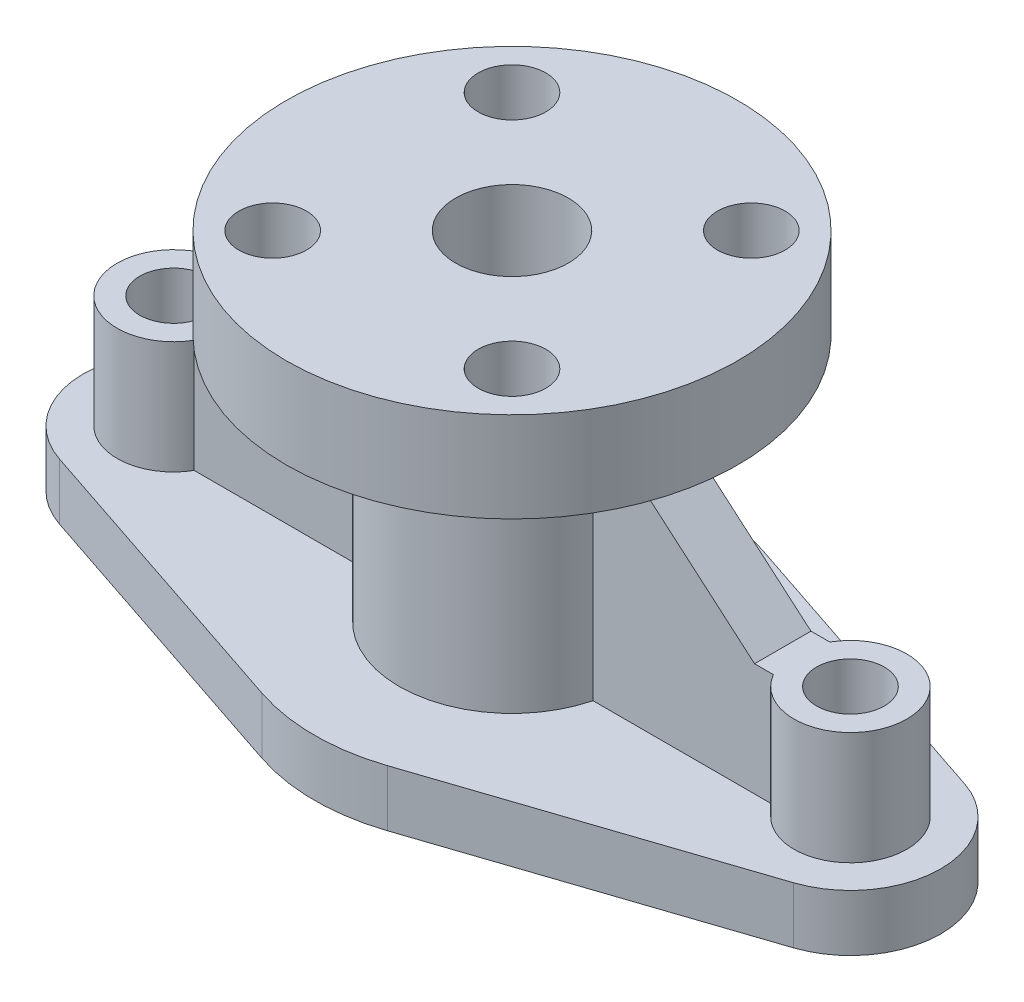
ISO-10303-21;
HEADER;
FILE_DESCRIPTION(('STEP AP214'),'2;1');
FILE_NAME('part.step','',(''),(''),'','','');
FILE_SCHEMA(('AUTOMOTIVE_DESIGN { 1 0 10303 214 1 1 1 1 }'));
ENDSEC;
DATA;
#1=APPLICATION_CONTEXT('core data for automotive mechanical design processes');
#2=APPLICATION_PROTOCOL_DEFINITION('international standard','automotive_design',2000,#1);
#3=PRODUCT_CONTEXT('',#1,'mechanical');
#4=PRODUCT('Part','Part','',(#3));
#5=PRODUCT_RELATED_PRODUCT_CATEGORY('part','',(#4));
#6=PRODUCT_DEFINITION_FORMATION('','',#4);
#7=PRODUCT_DEFINITION_CONTEXT('part definition',#1,'design');
#8=PRODUCT_DEFINITION('design','',#6,#7);
#9=PRODUCT_DEFINITION_SHAPE('','',#8);
#10=(LENGTH_UNIT() NAMED_UNIT(*) SI_UNIT(.MILLI.,.METRE.));
#11=(NAMED_UNIT(*) PLANE_ANGLE_UNIT() SI_UNIT($,.RADIAN.));
#12=(NAMED_UNIT(*) SI_UNIT($,.STERADIAN.) SOLID_ANGLE_UNIT());
#13=UNCERTAINTY_MEASURE_WITH_UNIT(LENGTH_MEASURE(1.E-05),#10,'distance_accuracy_value','');
#14=(GEOMETRIC_REPRESENTATION_CONTEXT(3) GLOBAL_UNCERTAINTY_ASSIGNED_CONTEXT((#13)) GLOBAL_UNIT_ASSIGNED_CONTEXT((#10,
#11,#12)) REPRESENTATION_CONTEXT('',''));
#15=CARTESIAN_POINT('',(0.,0.,0.));
#16=DIRECTION('',(0.,0.,1.));
#17=DIRECTION('',(1.,0.,0.));
#18=AXIS2_PLACEMENT_3D('',#15,#16,#17);
#19=CARTESIAN_POINT('',(0.,54.,0.));
#20=DIRECTION('',(0.,-1.,0.));
#21=DIRECTION('',(0.,0.,-1.));
#22=AXIS2_PLACEMENT_3D('',#19,#20,#21);
#23=CYLINDRICAL_SURFACE('',#22,20.);
#24=DIRECTION('',(0.,-1.,0.));
#25=VECTOR('',#24,1.);
#26=CARTESIAN_POINT('',(-19.3649167310371,54.,-5.));
#27=LINE('',#26,#25);
#28=CARTESIAN_POINT('',(-19.3649167310371,54.,-5.));
#29=VERTEX_POINT('',#28);
#30=CARTESIAN_POINT('',(-19.3649167310371,10.,-5.));
#31=VERTEX_POINT('',#30);
#32=EDGE_CURVE('E213',#29,#31,#27,.T.);
#33=ORIENTED_EDGE('',*,*,#32,.F.);
#34=CARTESIAN_POINT('',(0.,54.,0.));
#35=DIRECTION('',(0.,1.,0.));
#36=DIRECTION('',(0.,0.,1.));
#37=AXIS2_PLACEMENT_3D('',#34,#35,#36);
#38=CIRCLE('',#37,20.);
#39=CARTESIAN_POINT('',(19.3649167310371,54.,-5.));
#40=VERTEX_POINT('',#39);
#41=EDGE_CURVE('E311',#40,#29,#38,.T.);
#42=ORIENTED_EDGE('',*,*,#41,.F.);
#43=DIRECTION('',(0.,-1.,0.));
#44=VECTOR('',#43,1.);
#45=CARTESIAN_POINT('',(19.3649167310371,54.,-5.));
#46=LINE('',#45,#44);
#47=CARTESIAN_POINT('',(19.3649167310371,10.,-5.));
#48=VERTEX_POINT('',#47);
#49=EDGE_CURVE('E246',#48,#40,#46,.F.);
#50=ORIENTED_EDGE('',*,*,#49,.F.);
#51=CARTESIAN_POINT('',(0.,10.,0.));
#52=DIRECTION('',(0.,1.,0.));
#53=DIRECTION('',(0.,0.,1.));
#54=AXIS2_PLACEMENT_3D('',#51,#52,#53);
#55=CIRCLE('',#54,20.);
#56=EDGE_CURVE('E314',#48,#31,#55,.T.);
#57=ORIENTED_EDGE('',*,*,#56,.T.);
#58=EDGE_LOOP('',(#33,#42,#50,#57));
#59=FACE_BOUND('',#58,.T.);
#60=ADVANCED_FACE('F50',(#59),#23,.T.);
#61=CARTESIAN_POINT('',(-60.,10.,0.));
#62=DIRECTION('',(0.,-1.,0.));
#63=DIRECTION('',(0.,0.,-1.));
#64=AXIS2_PLACEMENT_3D('',#61,#62,#63);
#65=CYLINDRICAL_SURFACE('',#64,16.);
#66=DIRECTION('',(0.,-1.,0.));
#67=VECTOR('',#66,1.);
#68=CARTESIAN_POINT('',(-65.0666666666667,10.,15.176590160141));
#69=LINE('',#68,#67);
#70=CARTESIAN_POINT('',(-65.0666666666667,10.,15.176590160141));
#71=VERTEX_POINT('',#70);
#72=CARTESIAN_POINT('',(-65.0666666666667,0.,15.176590160141));
#73=VERTEX_POINT('',#72);
#74=EDGE_CURVE('E11',#71,#73,#69,.T.);
#75=ORIENTED_EDGE('',*,*,#74,.F.);
#76=CARTESIAN_POINT('',(-60.,10.,0.));
#77=DIRECTION('',(0.,1.,0.));
#78=DIRECTION('',(0.,0.,1.));
#79=AXIS2_PLACEMENT_3D('',#76,#77,#78);
#80=CIRCLE('',#79,16.);
#81=CARTESIAN_POINT('',(-65.0666666666667,10.,-15.176590160141));
#82=VERTEX_POINT('',#81);
#83=EDGE_CURVE('E337',#82,#71,#80,.T.);
#84=ORIENTED_EDGE('',*,*,#83,.F.);
#85=DIRECTION('',(0.,-1.,0.));
#86=VECTOR('',#85,1.);
#87=CARTESIAN_POINT('',(-65.0666666666667,10.,-15.176590160141));
#88=LINE('',#87,#86);
#89=CARTESIAN_POINT('',(-65.0666666666667,0.,-15.176590160141));
#90=VERTEX_POINT('',#89);
#91=EDGE_CURVE('E353',#82,#90,#88,.T.);
#92=ORIENTED_EDGE('',*,*,#91,.T.);
#93=CARTESIAN_POINT('',(-60.,0.,0.));
#94=DIRECTION('',(0.,1.,0.));
#95=DIRECTION('',(0.,0.,1.));
#96=AXIS2_PLACEMENT_3D('',#93,#94,#95);
#97=CIRCLE('',#96,16.);
#98=EDGE_CURVE('E332',#90,#73,#97,.T.);
#99=ORIENTED_EDGE('',*,*,#98,.T.);
#100=EDGE_LOOP('',(#75,#84,#92,#99));
#101=FACE_BOUND('',#100,.T.);
#102=ADVANCED_FACE('F47',(#101),#65,.T.);
#103=CARTESIAN_POINT('',(-65.0666666666667,10.,15.176590160141));
#104=DIRECTION('',(0.316666666666667,0.,-0.948536885008813));
#105=DIRECTION('',(-0.948536885008813,0.,-0.316666666666667));
#106=AXIS2_PLACEMENT_3D('',#103,#104,#105);
#107=PLANE('',#106);
#108=DIRECTION('',(0.948536885008813,0.,0.316666666666667));
#109=VECTOR('',#108,1.);
#110=CARTESIAN_POINT('',(-65.0666666666667,0.,15.176590160141));
#111=LINE('',#110,#109);
#112=CARTESIAN_POINT('',(-11.0833333333334,0.,33.1987909753084));
#113=VERTEX_POINT('',#112);
#114=EDGE_CURVE('E354',#73,#113,#111,.T.);
#115=ORIENTED_EDGE('',*,*,#114,.T.);
#116=DIRECTION('',(0.,-1.,0.));
#117=VECTOR('',#116,1.);
#118=CARTESIAN_POINT('',(-11.0833333333334,10.,33.1987909753084));
#119=LINE('',#118,#117);
#120=CARTESIAN_POINT('',(-11.0833333333334,10.,33.1987909753084));
#121=VERTEX_POINT('',#120);
#122=EDGE_CURVE('E54',#121,#113,#119,.T.);
#123=ORIENTED_EDGE('',*,*,#122,.F.);
#124=DIRECTION('',(0.948536885008813,0.,0.316666666666667));
#125=VECTOR('',#124,1.);
#126=CARTESIAN_POINT('',(-65.0666666666667,10.,15.176590160141));
#127=LINE('',#126,#125);
#128=EDGE_CURVE('E336',#71,#121,#127,.T.);
#129=ORIENTED_EDGE('',*,*,#128,.F.);
#130=ORIENTED_EDGE('',*,*,#74,.T.);
#131=EDGE_LOOP('',(#115,#123,#129,#130));
#132=FACE_BOUND('',#131,.T.);
#133=ADVANCED_FACE('F412',(#132),#107,.F.);
#134=CARTESIAN_POINT('',(0.,10.,0.));
#135=DIRECTION('',(0.,-1.,0.));
#136=DIRECTION('',(0.,0.,-1.));
#137=AXIS2_PLACEMENT_3D('',#134,#135,#136);
#138=CYLINDRICAL_SURFACE('',#137,35.);
#139=CARTESIAN_POINT('',(0.,0.,0.));
#140=DIRECTION('',(0.,1.,0.));
#141=DIRECTION('',(0.,0.,1.));
#142=AXIS2_PLACEMENT_3D('',#139,#140,#141);
#143=CIRCLE('',#142,35.);
#144=CARTESIAN_POINT('',(11.0833333333333,0.,33.1987909753085));
#145=VERTEX_POINT('',#144);
#146=EDGE_CURVE('E357',#113,#145,#143,.T.);
#147=ORIENTED_EDGE('',*,*,#146,.T.);
#148=DIRECTION('',(0.,-1.,0.));
#149=VECTOR('',#148,1.);
#150=CARTESIAN_POINT('',(11.0833333333333,10.,33.1987909753085));
#151=LINE('',#150,#149);
#152=CARTESIAN_POINT('',(11.0833333333333,10.,33.1987909753085));
#153=VERTEX_POINT('',#152);
#154=EDGE_CURVE('E385',#153,#145,#151,.T.);
#155=ORIENTED_EDGE('',*,*,#154,.F.);
#156=CARTESIAN_POINT('',(0.,10.,0.));
#157=DIRECTION('',(0.,1.,0.));
#158=DIRECTION('',(0.,0.,1.));
#159=AXIS2_PLACEMENT_3D('',#156,#157,#158);
#160=CIRCLE('',#159,35.);
#161=EDGE_CURVE('E344',#121,#153,#160,.T.);
#162=ORIENTED_EDGE('',*,*,#161,.F.);
#163=ORIENTED_EDGE('',*,*,#122,.T.);
#164=EDGE_LOOP('',(#147,#155,#162,#163));
#165=FACE_BOUND('',#164,.T.);
#166=ADVANCED_FACE('F388',(#165),#138,.T.);
#167=CARTESIAN_POINT('',(11.0833333333333,10.,33.1987909753085));
#168=DIRECTION('',(-0.316666666666667,0.,-0.948536885008813));
#169=DIRECTION('',(-0.948536885008813,0.,0.316666666666667));
#170=AXIS2_PLACEMENT_3D('',#167,#168,#169);
#171=PLANE('',#170);
#172=DIRECTION('',(0.948536885008813,0.,-0.316666666666667));
#173=VECTOR('',#172,1.);
#174=CARTESIAN_POINT('',(11.0833333333333,0.,33.1987909753085));
#175=LINE('',#174,#173);
#176=CARTESIAN_POINT('',(65.0666666666667,0.,15.176590160141));
#177=VERTEX_POINT('',#176);
#178=EDGE_CURVE('E360',#145,#177,#175,.T.);
#179=ORIENTED_EDGE('',*,*,#178,.T.);
#180=DIRECTION('',(0.,-1.,0.));
#181=VECTOR('',#180,1.);
#182=CARTESIAN_POINT('',(65.0666666666667,10.,15.176590160141));
#183=LINE('',#182,#181);
#184=CARTESIAN_POINT('',(65.0666666666667,10.,15.176590160141));
#185=VERTEX_POINT('',#184);
#186=EDGE_CURVE('E378',#185,#177,#183,.T.);
#187=ORIENTED_EDGE('',*,*,#186,.F.);
#188=DIRECTION('',(0.948536885008813,0.,-0.316666666666667));
#189=VECTOR('',#188,1.);
#190=CARTESIAN_POINT('',(11.0833333333333,10.,33.1987909753085));
#191=LINE('',#190,#189);
#192=EDGE_CURVE('E345',#153,#185,#191,.T.);
#193=ORIENTED_EDGE('',*,*,#192,.F.);
#194=ORIENTED_EDGE('',*,*,#154,.T.);
#195=EDGE_LOOP('',(#179,#187,#193,#194));
#196=FACE_BOUND('',#195,.T.);
#197=ADVANCED_FACE('F405',(#196),#171,.F.);
#198=CARTESIAN_POINT('',(60.,10.,0.));
#199=DIRECTION('',(0.,-1.,0.));
#200=DIRECTION('',(0.,0.,-1.));
#201=AXIS2_PLACEMENT_3D('',#198,#199,#200);
#202=CYLINDRICAL_SURFACE('',#201,16.);
#203=CARTESIAN_POINT('',(60.,0.,0.));
#204=DIRECTION('',(0.,1.,0.));
#205=DIRECTION('',(0.,0.,1.));
#206=AXIS2_PLACEMENT_3D('',#203,#204,#205);
#207=CIRCLE('',#206,16.);
#208=CARTESIAN_POINT('',(65.0666666666667,0.,-15.176590160141));
#209=VERTEX_POINT('',#208);
#210=EDGE_CURVE('E363',#177,#209,#207,.T.);
#211=ORIENTED_EDGE('',*,*,#210,.T.);
#212=DIRECTION('',(0.,-1.,0.));
#213=VECTOR('',#212,1.);
#214=CARTESIAN_POINT('',(65.0666666666667,10.,-15.176590160141));
#215=LINE('',#214,#213);
#216=CARTESIAN_POINT('',(65.0666666666667,10.,-15.176590160141));
#217=VERTEX_POINT('',#216);
#218=EDGE_CURVE('E376',#217,#209,#215,.T.);
#219=ORIENTED_EDGE('',*,*,#218,.F.);
#220=CARTESIAN_POINT('',(60.,10.,0.));
#221=DIRECTION('',(0.,1.,0.));
#222=DIRECTION('',(0.,0.,1.));
#223=AXIS2_PLACEMENT_3D('',#220,#221,#222);
#224=CIRCLE('',#223,16.);
#225=EDGE_CURVE('E342',#185,#217,#224,.T.);
#226=ORIENTED_EDGE('',*,*,#225,.F.);
#227=ORIENTED_EDGE('',*,*,#186,.T.);
#228=EDGE_LOOP('',(#211,#219,#226,#227));
#229=FACE_BOUND('',#228,.T.);
#230=ADVANCED_FACE('F409',(#229),#202,.T.);
#231=CARTESIAN_POINT('',(65.0666666666667,10.,-15.176590160141));
#232=DIRECTION('',(-0.316666666666667,0.,0.948536885008813));
#233=DIRECTION('',(0.948536885008813,0.,0.316666666666667));
#234=AXIS2_PLACEMENT_3D('',#231,#232,#233);
#235=PLANE('',#234);
#236=DIRECTION('',(-0.948536885008813,0.,-0.316666666666667));
#237=VECTOR('',#236,1.);
#238=CARTESIAN_POINT('',(65.0666666666667,0.,-15.176590160141));
#239=LINE('',#238,#237);
#240=CARTESIAN_POINT('',(11.0833333333333,0.,-33.1987909753085));
#241=VERTEX_POINT('',#240);
#242=EDGE_CURVE('E361',#209,#241,#239,.T.);
#243=ORIENTED_EDGE('',*,*,#242,.T.);
#244=DIRECTION('',(0.,-1.,0.));
#245=VECTOR('',#244,1.);
#246=CARTESIAN_POINT('',(11.0833333333333,10.,-33.1987909753085));
#247=LINE('',#246,#245);
#248=CARTESIAN_POINT('',(11.0833333333333,10.,-33.1987909753085));
#249=VERTEX_POINT('',#248);
#250=EDGE_CURVE('E373',#249,#241,#247,.T.);
#251=ORIENTED_EDGE('',*,*,#250,.F.);
#252=DIRECTION('',(-0.948536885008813,0.,-0.316666666666667));
#253=VECTOR('',#252,1.);
#254=CARTESIAN_POINT('',(65.0666666666667,10.,-15.176590160141));
#255=LINE('',#254,#253);
#256=EDGE_CURVE('E350',#217,#249,#255,.T.);
#257=ORIENTED_EDGE('',*,*,#256,.F.);
#258=ORIENTED_EDGE('',*,*,#218,.T.);
#259=EDGE_LOOP('',(#243,#251,#257,#258));
#260=FACE_BOUND('',#259,.T.);
#261=ADVANCED_FACE('F430',(#260),#235,.F.);
#262=CARTESIAN_POINT('',(0.,10.,0.));
#263=DIRECTION('',(0.,-1.,0.));
#264=DIRECTION('',(0.,0.,-1.));
#265=AXIS2_PLACEMENT_3D('',#262,#263,#264);
#266=CYLINDRICAL_SURFACE('',#265,35.);
#267=CARTESIAN_POINT('',(0.,0.,0.));
#268=DIRECTION('',(0.,1.,0.));
#269=DIRECTION('',(0.,0.,1.));
#270=AXIS2_PLACEMENT_3D('',#267,#268,#269);
#271=CIRCLE('',#270,35.);
#272=CARTESIAN_POINT('',(-11.0833333333333,0.,-33.1987909753085));
#273=VERTEX_POINT('',#272);
#274=EDGE_CURVE('E362',#241,#273,#271,.T.);
#275=ORIENTED_EDGE('',*,*,#274,.T.);
#276=DIRECTION('',(0.,-1.,0.));
#277=VECTOR('',#276,1.);
#278=CARTESIAN_POINT('',(-11.0833333333333,10.,-33.1987909753085));
#279=LINE('',#278,#277);
#280=CARTESIAN_POINT('',(-11.0833333333333,10.,-33.1987909753085));
#281=VERTEX_POINT('',#280);
#282=EDGE_CURVE('E369',#281,#273,#279,.T.);
#283=ORIENTED_EDGE('',*,*,#282,.F.);
#284=CARTESIAN_POINT('',(0.,10.,0.));
#285=DIRECTION('',(0.,1.,0.));
#286=DIRECTION('',(0.,0.,1.));
#287=AXIS2_PLACEMENT_3D('',#284,#285,#286);
#288=CIRCLE('',#287,35.);
#289=EDGE_CURVE('E347',#249,#281,#288,.T.);
#290=ORIENTED_EDGE('',*,*,#289,.F.);
#291=ORIENTED_EDGE('',*,*,#250,.T.);
#292=EDGE_LOOP('',(#275,#283,#290,#291));
#293=FACE_BOUND('',#292,.T.);
#294=ADVANCED_FACE('F424',(#293),#266,.T.);
#295=CARTESIAN_POINT('',(-65.0666666666667,10.,-15.176590160141));
#296=DIRECTION('',(0.316666666666666,0.,0.948536885008813));
#297=DIRECTION('',(0.948536885008813,0.,-0.316666666666666));
#298=AXIS2_PLACEMENT_3D('',#295,#296,#297);
#299=PLANE('',#298);
#300=DIRECTION('',(-0.948536885008813,0.,0.316666666666666));
#301=VECTOR('',#300,1.);
#302=CARTESIAN_POINT('',(-65.0666666666667,0.,-15.176590160141));
#303=LINE('',#302,#301);
#304=EDGE_CURVE('E339',#273,#90,#303,.T.);
#305=ORIENTED_EDGE('',*,*,#304,.T.);
#306=ORIENTED_EDGE('',*,*,#91,.F.);
#307=DIRECTION('',(-0.948536885008813,0.,0.316666666666666));
#308=VECTOR('',#307,1.);
#309=CARTESIAN_POINT('',(-65.0666666666667,10.,-15.176590160141));
#310=LINE('',#309,#308);
#311=EDGE_CURVE('E351',#281,#82,#310,.T.);
#312=ORIENTED_EDGE('',*,*,#311,.F.);
#313=ORIENTED_EDGE('',*,*,#282,.T.);
#314=EDGE_LOOP('',(#305,#306,#312,#313));
#315=FACE_BOUND('',#314,.T.);
#316=ADVANCED_FACE('F419',(#315),#299,.F.);
#317=CARTESIAN_POINT('',(-60.,10.,0.));
#318=DIRECTION('',(0.,1.,0.));
#319=DIRECTION('',(0.,0.,1.));
#320=AXIS2_PLACEMENT_3D('',#317,#318,#319);
#321=PLANE('',#320);
#322=DIRECTION('',(1.,0.,0.));
#323=VECTOR('',#322,1.);
#324=CARTESIAN_POINT('',(-60.,10.,5.));
#325=LINE('',#324,#323);
#326=CARTESIAN_POINT('',(-51.3397459621556,10.,5.));
#327=VERTEX_POINT('',#326);
#328=CARTESIAN_POINT('',(-19.3649167310371,10.,5.));
#329=VERTEX_POINT('',#328);
#330=EDGE_CURVE('E223',#327,#329,#325,.T.);
#331=ORIENTED_EDGE('',*,*,#330,.F.);
#332=CARTESIAN_POINT('',(-60.,10.,0.));
#333=DIRECTION('',(0.,1.,0.));
#334=DIRECTION('',(0.,0.,1.));
#335=AXIS2_PLACEMENT_3D('',#332,#333,#334);
#336=CIRCLE('',#335,10.);
#337=CARTESIAN_POINT('',(-51.3397459621556,10.,-5.));
#338=VERTEX_POINT('',#337);
#339=EDGE_CURVE('E66',#338,#327,#336,.T.);
#340=ORIENTED_EDGE('',*,*,#339,.F.);
#341=DIRECTION('',(1.,0.,0.));
#342=VECTOR('',#341,1.);
#343=CARTESIAN_POINT('',(-60.,10.,-5.));
#344=LINE('',#343,#342);
#345=EDGE_CURVE('E220',#338,#31,#344,.T.);
#346=ORIENTED_EDGE('',*,*,#345,.T.);
#347=ORIENTED_EDGE('',*,*,#56,.F.);
#348=DIRECTION('',(1.,0.,0.));
#349=VECTOR('',#348,1.);
#350=CARTESIAN_POINT('',(-60.,10.,-5.));
#351=LINE('',#350,#349);
#352=CARTESIAN_POINT('',(51.3397459621556,10.,-5.));
#353=VERTEX_POINT('',#352);
#354=EDGE_CURVE('E250',#48,#353,#351,.T.);
#355=ORIENTED_EDGE('',*,*,#354,.T.);
#356=CARTESIAN_POINT('',(60.,10.,0.));
#357=DIRECTION('',(0.,1.,0.));
#358=DIRECTION('',(0.,0.,1.));
#359=AXIS2_PLACEMENT_3D('',#356,#357,#358);
#360=CIRCLE('',#359,9.99999999999999);
#361=CARTESIAN_POINT('',(51.3397459621556,10.,5.));
#362=VERTEX_POINT('',#361);
#363=EDGE_CURVE('E327',#362,#353,#360,.T.);
#364=ORIENTED_EDGE('',*,*,#363,.F.);
#365=DIRECTION('',(1.,0.,0.));
#366=VECTOR('',#365,1.);
#367=CARTESIAN_POINT('',(-60.,10.,5.));
#368=LINE('',#367,#366);
#369=CARTESIAN_POINT('',(19.3649167310371,10.,5.));
#370=VERTEX_POINT('',#369);
#371=EDGE_CURVE('E260',#370,#362,#368,.T.);
#372=ORIENTED_EDGE('',*,*,#371,.F.);
#373=EDGE_CURVE('E308',#329,#370,#55,.T.);
#374=ORIENTED_EDGE('',*,*,#373,.F.);
#375=EDGE_LOOP('',(#331,#340,#346,#347,#355,#364,#372,#374));
#376=FACE_BOUND('',#375,.T.);
#377=ORIENTED_EDGE('',*,*,#83,.T.);
#378=ORIENTED_EDGE('',*,*,#128,.T.);
#379=ORIENTED_EDGE('',*,*,#161,.T.);
#380=ORIENTED_EDGE('',*,*,#192,.T.);
#381=ORIENTED_EDGE('',*,*,#225,.T.);
#382=ORIENTED_EDGE('',*,*,#256,.T.);
#383=ORIENTED_EDGE('',*,*,#289,.T.);
#384=ORIENTED_EDGE('',*,*,#311,.T.);
#385=EDGE_LOOP('',(#377,#378,#379,#380,#381,#382,#383,#384));
#386=FACE_BOUND('',#385,.T.);
#387=ADVANCED_FACE('F407',(#376,#386),#321,.T.);
#388=CARTESIAN_POINT('',(-60.,0.,0.));
#389=DIRECTION('',(0.,1.,0.));
#390=DIRECTION('',(0.,0.,1.));
#391=AXIS2_PLACEMENT_3D('',#388,#389,#390);
#392=PLANE('',#391);
#393=CARTESIAN_POINT('',(-60.,0.,0.));
#394=DIRECTION('',(0.,1.,0.));
#395=DIRECTION('',(0.,0.,1.));
#396=AXIS2_PLACEMENT_3D('',#393,#394,#395);
#397=CIRCLE('',#396,6.);
#398=CARTESIAN_POINT('',(-60.,0.,6.));
#399=VERTEX_POINT('',#398);
#400=EDGE_CURVE('E319',#399,#399,#397,.T.);
#401=ORIENTED_EDGE('',*,*,#400,.T.);
#402=EDGE_LOOP('',(#401));
#403=FACE_BOUND('',#402,.T.);
#404=CARTESIAN_POINT('',(0.,0.,0.));
#405=DIRECTION('',(0.,1.,0.));
#406=DIRECTION('',(0.,0.,1.));
#407=AXIS2_PLACEMENT_3D('',#404,#405,#406);
#408=CIRCLE('',#407,5.);
#409=CARTESIAN_POINT('',(0.,0.,5.));
#410=VERTEX_POINT('',#409);
#411=EDGE_CURVE('E268',#410,#410,#408,.T.);
#412=ORIENTED_EDGE('',*,*,#411,.T.);
#413=EDGE_LOOP('',(#412));
#414=FACE_BOUND('',#413,.T.);
#415=CARTESIAN_POINT('',(60.,0.,0.));
#416=DIRECTION('',(0.,1.,0.));
#417=DIRECTION('',(0.,0.,1.));
#418=AXIS2_PLACEMENT_3D('',#415,#416,#417);
#419=CIRCLE('',#418,6.);
#420=CARTESIAN_POINT('',(60.,0.,6.));
#421=VERTEX_POINT('',#420);
#422=EDGE_CURVE('E326',#421,#421,#419,.T.);
#423=ORIENTED_EDGE('',*,*,#422,.T.);
#424=EDGE_LOOP('',(#423));
#425=FACE_BOUND('',#424,.T.);
#426=ORIENTED_EDGE('',*,*,#114,.F.);
#427=ORIENTED_EDGE('',*,*,#98,.F.);
#428=ORIENTED_EDGE('',*,*,#304,.F.);
#429=ORIENTED_EDGE('',*,*,#274,.F.);
#430=ORIENTED_EDGE('',*,*,#242,.F.);
#431=ORIENTED_EDGE('',*,*,#210,.F.);
#432=ORIENTED_EDGE('',*,*,#178,.F.);
#433=ORIENTED_EDGE('',*,*,#146,.F.);
#434=EDGE_LOOP('',(#426,#427,#428,#429,#430,#431,#432,#433));
#435=FACE_BOUND('',#434,.T.);
#436=ADVANCED_FACE('F396',(#403,#414,#425,#435),#392,.F.);
#437=CARTESIAN_POINT('',(60.,30.,0.));
#438=DIRECTION('',(0.,-1.,0.));
#439=DIRECTION('',(0.,0.,-1.));
#440=AXIS2_PLACEMENT_3D('',#437,#438,#439);
#441=CYLINDRICAL_SURFACE('',#440,9.99999999999999);
#442=ORIENTED_EDGE('',*,*,#363,.T.);
#443=DIRECTION('',(0.,-1.,0.));
#444=VECTOR('',#443,1.);
#445=CARTESIAN_POINT('',(51.3397459621556,30.,-5.));
#446=LINE('',#445,#444);
#447=CARTESIAN_POINT('',(51.3397459621556,30.,-5.));
#448=VERTEX_POINT('',#447);
#449=EDGE_CURVE('E249',#448,#353,#446,.T.);
#450=ORIENTED_EDGE('',*,*,#449,.F.);
#451=CARTESIAN_POINT('',(60.,30.,0.));
#452=DIRECTION('',(0.,1.,0.));
#453=DIRECTION('',(0.,0.,1.));
#454=AXIS2_PLACEMENT_3D('',#451,#452,#453);
#455=CIRCLE('',#454,9.99999999999999);
#456=CARTESIAN_POINT('',(51.3397459621556,30.,5.));
#457=VERTEX_POINT('',#456);
#458=EDGE_CURVE('E335',#457,#448,#455,.T.);
#459=ORIENTED_EDGE('',*,*,#458,.F.);
#460=DIRECTION('',(0.,-1.,0.));
#461=VECTOR('',#460,1.);
#462=CARTESIAN_POINT('',(51.3397459621556,30.,5.));
#463=LINE('',#462,#461);
#464=EDGE_CURVE('E261',#457,#362,#463,.T.);
#465=ORIENTED_EDGE('',*,*,#464,.T.);
#466=EDGE_LOOP('',(#442,#450,#459,#465));
#467=FACE_BOUND('',#466,.T.);
#468=ADVANCED_FACE('F489',(#467),#441,.T.);
#469=CARTESIAN_POINT('',(60.,30.,0.));
#470=DIRECTION('',(0.,1.,0.));
#471=DIRECTION('',(0.,0.,1.));
#472=AXIS2_PLACEMENT_3D('',#469,#470,#471);
#473=PLANE('',#472);
#474=CARTESIAN_POINT('',(60.,30.,0.));
#475=DIRECTION('',(0.,1.,0.));
#476=DIRECTION('',(0.,0.,1.));
#477=AXIS2_PLACEMENT_3D('',#474,#475,#476);
#478=CIRCLE('',#477,6.);
#479=CARTESIAN_POINT('',(60.,30.,6.));
#480=VERTEX_POINT('',#479);
#481=EDGE_CURVE('E323',#480,#480,#478,.T.);
#482=ORIENTED_EDGE('',*,*,#481,.F.);
#483=EDGE_LOOP('',(#482));
#484=FACE_BOUND('',#483,.T.);
#485=DIRECTION('',(1.,0.,0.));
#486=VECTOR('',#485,1.);
#487=CARTESIAN_POINT('',(0.,30.,5.));
#488=LINE('',#487,#486);
#489=CARTESIAN_POINT('',(48.,30.,5.));
#490=VERTEX_POINT('',#489);
#491=EDGE_CURVE('E233',#490,#457,#488,.T.);
#492=ORIENTED_EDGE('',*,*,#491,.T.);
#493=ORIENTED_EDGE('',*,*,#458,.T.);
#494=DIRECTION('',(1.,0.,0.));
#495=VECTOR('',#494,1.);
#496=CARTESIAN_POINT('',(0.,30.,-5.));
#497=LINE('',#496,#495);
#498=CARTESIAN_POINT('',(48.,30.,-5.));
#499=VERTEX_POINT('',#498);
#500=EDGE_CURVE('E240',#499,#448,#497,.T.);
#501=ORIENTED_EDGE('',*,*,#500,.F.);
#502=DIRECTION('',(0.,0.,1.));
#503=VECTOR('',#502,1.);
#504=CARTESIAN_POINT('',(48.,30.,0.));
#505=LINE('',#504,#503);
#506=EDGE_CURVE('E234',#499,#490,#505,.T.);
#507=ORIENTED_EDGE('',*,*,#506,.T.);
#508=EDGE_LOOP('',(#492,#493,#501,#507));
#509=FACE_BOUND('',#508,.T.);
#510=ADVANCED_FACE('F495',(#484,#509),#473,.T.);
#511=CARTESIAN_POINT('',(60.,0.,0.));
#512=DIRECTION('',(0.,1.,0.));
#513=DIRECTION('',(0.,0.,1.));
#514=AXIS2_PLACEMENT_3D('',#511,#512,#513);
#515=CYLINDRICAL_SURFACE('',#514,6.);
#516=ORIENTED_EDGE('',*,*,#422,.F.);
#517=EDGE_LOOP('',(#516));
#518=FACE_BOUND('',#517,.T.);
#519=ORIENTED_EDGE('',*,*,#481,.T.);
#520=EDGE_LOOP('',(#519));
#521=FACE_BOUND('',#520,.T.);
#522=ADVANCED_FACE('F494',(#518,#521),#515,.F.);
#523=CARTESIAN_POINT('',(-60.,30.,0.));
#524=DIRECTION('',(0.,-1.,0.));
#525=DIRECTION('',(0.,0.,-1.));
#526=AXIS2_PLACEMENT_3D('',#523,#524,#525);
#527=CYLINDRICAL_SURFACE('',#526,10.);
#528=DIRECTION('',(0.,-1.,0.));
#529=VECTOR('',#528,1.);
#530=CARTESIAN_POINT('',(-51.3397459621556,30.,5.));
#531=LINE('',#530,#529);
#532=CARTESIAN_POINT('',(-51.3397459621556,30.,5.));
#533=VERTEX_POINT('',#532);
#534=EDGE_CURVE('E228',#327,#533,#531,.F.);
#535=ORIENTED_EDGE('',*,*,#534,.T.);
#536=CARTESIAN_POINT('',(-60.,30.,0.));
#537=DIRECTION('',(0.,1.,0.));
#538=DIRECTION('',(0.,0.,1.));
#539=AXIS2_PLACEMENT_3D('',#536,#537,#538);
#540=CIRCLE('',#539,10.);
#541=CARTESIAN_POINT('',(-51.3397459621556,30.,-5.));
#542=VERTEX_POINT('',#541);
#543=EDGE_CURVE('E210',#542,#533,#540,.T.);
#544=ORIENTED_EDGE('',*,*,#543,.F.);
#545=DIRECTION('',(0.,-1.,0.));
#546=VECTOR('',#545,1.);
#547=CARTESIAN_POINT('',(-51.3397459621556,30.,-5.));
#548=LINE('',#547,#546);
#549=EDGE_CURVE('E61',#338,#542,#548,.F.);
#550=ORIENTED_EDGE('',*,*,#549,.F.);
#551=ORIENTED_EDGE('',*,*,#339,.T.);
#552=EDGE_LOOP('',(#535,#544,#550,#551));
#553=FACE_BOUND('',#552,.T.);
#554=ADVANCED_FACE('F505',(#553),#527,.T.);
#555=CARTESIAN_POINT('',(-60.,30.,0.));
#556=DIRECTION('',(0.,1.,0.));
#557=DIRECTION('',(0.,0.,1.));
#558=AXIS2_PLACEMENT_3D('',#555,#556,#557);
#559=PLANE('',#558);
#560=CARTESIAN_POINT('',(-60.,30.,0.));
#561=DIRECTION('',(0.,1.,0.));
#562=DIRECTION('',(0.,0.,1.));
#563=AXIS2_PLACEMENT_3D('',#560,#561,#562);
#564=CIRCLE('',#563,6.);
#565=CARTESIAN_POINT('',(-60.,30.,6.));
#566=VERTEX_POINT('',#565);
#567=EDGE_CURVE('E312',#566,#566,#564,.T.);
#568=ORIENTED_EDGE('',*,*,#567,.F.);
#569=EDGE_LOOP('',(#568));
#570=FACE_BOUND('',#569,.T.);
#571=ORIENTED_EDGE('',*,*,#543,.T.);
#572=DIRECTION('',(1.,0.,0.));
#573=VECTOR('',#572,1.);
#574=CARTESIAN_POINT('',(0.,30.,5.));
#575=LINE('',#574,#573);
#576=CARTESIAN_POINT('',(-48.,30.,5.));
#577=VERTEX_POINT('',#576);
#578=EDGE_CURVE('E186',#577,#533,#575,.F.);
#579=ORIENTED_EDGE('',*,*,#578,.F.);
#580=DIRECTION('',(0.,0.,1.));
#581=VECTOR('',#580,1.);
#582=CARTESIAN_POINT('',(-48.,30.,0.));
#583=LINE('',#582,#581);
#584=CARTESIAN_POINT('',(-48.,30.,-5.));
#585=VERTEX_POINT('',#584);
#586=EDGE_CURVE('E200',#585,#577,#583,.T.);
#587=ORIENTED_EDGE('',*,*,#586,.F.);
#588=DIRECTION('',(1.,0.,0.));
#589=VECTOR('',#588,1.);
#590=CARTESIAN_POINT('',(0.,30.,-5.));
#591=LINE('',#590,#589);
#592=EDGE_CURVE('E193',#585,#542,#591,.F.);
#593=ORIENTED_EDGE('',*,*,#592,.T.);
#594=EDGE_LOOP('',(#571,#579,#587,#593));
#595=FACE_BOUND('',#594,.T.);
#596=ADVANCED_FACE('F207',(#570,#595),#559,.T.);
#597=CARTESIAN_POINT('',(-60.,0.,0.));
#598=DIRECTION('',(0.,1.,0.));
#599=DIRECTION('',(0.,0.,1.));
#600=AXIS2_PLACEMENT_3D('',#597,#598,#599);
#601=CYLINDRICAL_SURFACE('',#600,6.);
#602=ORIENTED_EDGE('',*,*,#400,.F.);
#603=EDGE_LOOP('',(#602));
#604=FACE_BOUND('',#603,.T.);
#605=ORIENTED_EDGE('',*,*,#567,.T.);
#606=EDGE_LOOP('',(#605));
#607=FACE_BOUND('',#606,.T.);
#608=ADVANCED_FACE('F448',(#604,#607),#601,.F.);
#609=CARTESIAN_POINT('',(-19.3649167310371,54.,5.));
#610=VERTEX_POINT('',#609);
#611=CARTESIAN_POINT('',(19.3649167310371,54.,5.));
#612=VERTEX_POINT('',#611);
#613=EDGE_CURVE('E313',#610,#612,#38,.T.);
#614=ORIENTED_EDGE('',*,*,#613,.F.);
#615=DIRECTION('',(0.,-1.,0.));
#616=VECTOR('',#615,1.);
#617=CARTESIAN_POINT('',(-19.3649167310371,54.,5.));
#618=LINE('',#617,#616);
#619=EDGE_CURVE('E221',#610,#329,#618,.T.);
#620=ORIENTED_EDGE('',*,*,#619,.T.);
#621=ORIENTED_EDGE('',*,*,#373,.T.);
#622=DIRECTION('',(0.,-1.,0.));
#623=VECTOR('',#622,1.);
#624=CARTESIAN_POINT('',(19.3649167310371,54.,5.));
#625=LINE('',#624,#623);
#626=EDGE_CURVE('E256',#370,#612,#625,.F.);
#627=ORIENTED_EDGE('',*,*,#626,.T.);
#628=EDGE_LOOP('',(#614,#620,#621,#627));
#629=FACE_BOUND('',#628,.T.);
#630=ADVANCED_FACE('F439',(#629),#23,.T.);
#631=CARTESIAN_POINT('',(0.,70.,0.));
#632=DIRECTION('',(0.,-1.,0.));
#633=DIRECTION('',(0.,0.,-1.));
#634=AXIS2_PLACEMENT_3D('',#631,#632,#633);
#635=CYLINDRICAL_SURFACE('',#634,40.);
#636=CARTESIAN_POINT('',(0.,70.,0.));
#637=DIRECTION('',(0.,1.,0.));
#638=DIRECTION('',(0.,0.,1.));
#639=AXIS2_PLACEMENT_3D('',#636,#637,#638);
#640=CIRCLE('',#639,40.);
#641=CARTESIAN_POINT('',(0.,70.,40.));
#642=VERTEX_POINT('',#641);
#643=EDGE_CURVE('E304',#642,#642,#640,.T.);
#644=ORIENTED_EDGE('',*,*,#643,.F.);
#645=EDGE_LOOP('',(#644));
#646=FACE_BOUND('',#645,.T.);
#647=CARTESIAN_POINT('',(0.,54.,0.));
#648=DIRECTION('',(0.,1.,0.));
#649=DIRECTION('',(0.,0.,1.));
#650=AXIS2_PLACEMENT_3D('',#647,#648,#649);
#651=CIRCLE('',#650,40.);
#652=CARTESIAN_POINT('',(0.,54.,40.));
#653=VERTEX_POINT('',#652);
#654=EDGE_CURVE('E305',#653,#653,#651,.T.);
#655=ORIENTED_EDGE('',*,*,#654,.T.);
#656=EDGE_LOOP('',(#655));
#657=FACE_BOUND('',#656,.T.);
#658=ADVANCED_FACE('F446',(#646,#657),#635,.T.);
#659=CARTESIAN_POINT('',(0.,70.,0.));
#660=DIRECTION('',(0.,1.,0.));
#661=DIRECTION('',(0.,0.,1.));
#662=AXIS2_PLACEMENT_3D('',#659,#660,#661);
#663=PLANE('',#662);
#664=ORIENTED_EDGE('',*,*,#643,.T.);
#665=EDGE_LOOP('',(#664));
#666=FACE_BOUND('',#665,.T.);
#667=CARTESIAN_POINT('',(0.,70.,0.));
#668=DIRECTION('',(0.,1.,0.));
#669=DIRECTION('',(0.,0.,1.));
#670=AXIS2_PLACEMENT_3D('',#667,#668,#669);
#671=CIRCLE('',#670,10.);
#672=CARTESIAN_POINT('',(0.,70.,10.));
#673=VERTEX_POINT('',#672);
#674=EDGE_CURVE('E276',#673,#673,#671,.T.);
#675=ORIENTED_EDGE('',*,*,#674,.F.);
#676=EDGE_LOOP('',(#675));
#677=FACE_BOUND('',#676,.T.);
#678=CARTESIAN_POINT('',(-21.2132034355965,70.,-21.2132034355963));
#679=DIRECTION('',(0.,1.,0.));
#680=DIRECTION('',(0.,0.,1.));
#681=AXIS2_PLACEMENT_3D('',#678,#679,#680);
#682=CIRCLE('',#681,6.);
#683=CARTESIAN_POINT('',(-21.2132034355965,70.,-15.2132034355963));
#684=VERTEX_POINT('',#683);
#685=EDGE_CURVE('E295',#684,#684,#682,.T.);
#686=ORIENTED_EDGE('',*,*,#685,.F.);
#687=EDGE_LOOP('',(#686));
#688=FACE_BOUND('',#687,.T.);
#689=CARTESIAN_POINT('',(-21.2132034355965,70.,21.2132034355963));
#690=DIRECTION('',(0.,1.,0.));
#691=DIRECTION('',(0.,0.,1.));
#692=AXIS2_PLACEMENT_3D('',#689,#690,#691);
#693=CIRCLE('',#692,6.);
#694=CARTESIAN_POINT('',(-21.2132034355965,70.,27.2132034355963));
#695=VERTEX_POINT('',#694);
#696=EDGE_CURVE('E288',#695,#695,#693,.T.);
#697=ORIENTED_EDGE('',*,*,#696,.F.);
#698=EDGE_LOOP('',(#697));
#699=FACE_BOUND('',#698,.T.);
#700=CARTESIAN_POINT('',(21.2132034355965,70.,21.2132034355964));
#701=DIRECTION('',(0.,1.,0.));
#702=DIRECTION('',(0.,0.,1.));
#703=AXIS2_PLACEMENT_3D('',#700,#701,#702);
#704=CIRCLE('',#703,6.);
#705=CARTESIAN_POINT('',(21.2132034355965,70.,27.2132034355964));
#706=VERTEX_POINT('',#705);
#707=EDGE_CURVE('E281',#706,#706,#704,.T.);
#708=ORIENTED_EDGE('',*,*,#707,.F.);
#709=EDGE_LOOP('',(#708));
#710=FACE_BOUND('',#709,.T.);
#711=CARTESIAN_POINT('',(21.2132034355964,70.,-21.2132034355965));
#712=DIRECTION('',(0.,1.,0.));
#713=DIRECTION('',(0.,0.,1.));
#714=AXIS2_PLACEMENT_3D('',#711,#712,#713);
#715=CIRCLE('',#714,6.);
#716=CARTESIAN_POINT('',(21.2132034355964,70.,-15.2132034355965));
#717=VERTEX_POINT('',#716);
#718=EDGE_CURVE('E282',#717,#717,#715,.T.);
#719=ORIENTED_EDGE('',*,*,#718,.F.);
#720=EDGE_LOOP('',(#719));
#721=FACE_BOUND('',#720,.T.);
#722=ADVANCED_FACE('F456',(#666,#677,#688,#699,#710,#721),#663,.T.);
#723=CARTESIAN_POINT('',(0.,54.,0.));
#724=DIRECTION('',(0.,1.,0.));
#725=DIRECTION('',(0.,0.,1.));
#726=AXIS2_PLACEMENT_3D('',#723,#724,#725);
#727=PLANE('',#726);
#728=ORIENTED_EDGE('',*,*,#654,.F.);
#729=EDGE_LOOP('',(#728));
#730=FACE_BOUND('',#729,.T.);
#731=DIRECTION('',(1.,0.,0.));
#732=VECTOR('',#731,1.);
#733=CARTESIAN_POINT('',(0.,54.,5.));
#734=LINE('',#733,#732);
#735=CARTESIAN_POINT('',(20.,54.,5.));
#736=VERTEX_POINT('',#735);
#737=EDGE_CURVE('E253',#612,#736,#734,.T.);
#738=ORIENTED_EDGE('',*,*,#737,.T.);
#739=DIRECTION('',(0.,0.,1.));
#740=VECTOR('',#739,1.);
#741=CARTESIAN_POINT('',(20.,54.,0.));
#742=LINE('',#741,#740);
#743=CARTESIAN_POINT('',(20.,54.,-5.));
#744=VERTEX_POINT('',#743);
#745=EDGE_CURVE('E266',#736,#744,#742,.F.);
#746=ORIENTED_EDGE('',*,*,#745,.T.);
#747=DIRECTION('',(1.,0.,0.));
#748=VECTOR('',#747,1.);
#749=CARTESIAN_POINT('',(0.,54.,-5.));
#750=LINE('',#749,#748);
#751=EDGE_CURVE('E243',#40,#744,#750,.T.);
#752=ORIENTED_EDGE('',*,*,#751,.F.);
#753=ORIENTED_EDGE('',*,*,#41,.T.);
#754=DIRECTION('',(1.,0.,0.));
#755=VECTOR('',#754,1.);
#756=CARTESIAN_POINT('',(0.,54.,-5.));
#757=LINE('',#756,#755);
#758=CARTESIAN_POINT('',(-20.,54.,-5.));
#759=VERTEX_POINT('',#758);
#760=EDGE_CURVE('E202',#759,#29,#757,.T.);
#761=ORIENTED_EDGE('',*,*,#760,.F.);
#762=DIRECTION('',(0.,0.,1.));
#763=VECTOR('',#762,1.);
#764=CARTESIAN_POINT('',(-20.,54.,0.));
#765=LINE('',#764,#763);
#766=CARTESIAN_POINT('',(-20.,54.,5.));
#767=VERTEX_POINT('',#766);
#768=EDGE_CURVE('E226',#759,#767,#765,.T.);
#769=ORIENTED_EDGE('',*,*,#768,.T.);
#770=DIRECTION('',(1.,0.,0.));
#771=VECTOR('',#770,1.);
#772=CARTESIAN_POINT('',(0.,54.,5.));
#773=LINE('',#772,#771);
#774=EDGE_CURVE('E194',#767,#610,#773,.T.);
#775=ORIENTED_EDGE('',*,*,#774,.T.);
#776=ORIENTED_EDGE('',*,*,#613,.T.);
#777=EDGE_LOOP('',(#738,#746,#752,#753,#761,#769,#775,#776));
#778=FACE_BOUND('',#777,.T.);
#779=CARTESIAN_POINT('',(-21.2132034355965,54.,-21.2132034355963));
#780=DIRECTION('',(0.,1.,0.));
#781=DIRECTION('',(0.,0.,1.));
#782=AXIS2_PLACEMENT_3D('',#779,#780,#781);
#783=CIRCLE('',#782,6.);
#784=CARTESIAN_POINT('',(-21.2132034355965,54.,-15.2132034355963));
#785=VERTEX_POINT('',#784);
#786=EDGE_CURVE('E277',#785,#785,#783,.T.);
#787=ORIENTED_EDGE('',*,*,#786,.T.);
#788=EDGE_LOOP('',(#787));
#789=FACE_BOUND('',#788,.T.);
#790=CARTESIAN_POINT('',(-21.2132034355965,54.,21.2132034355963));
#791=DIRECTION('',(0.,1.,0.));
#792=DIRECTION('',(0.,0.,1.));
#793=AXIS2_PLACEMENT_3D('',#790,#791,#792);
#794=CIRCLE('',#793,6.);
#795=CARTESIAN_POINT('',(-21.2132034355965,54.,27.2132034355963));
#796=VERTEX_POINT('',#795);
#797=EDGE_CURVE('E293',#796,#796,#794,.T.);
#798=ORIENTED_EDGE('',*,*,#797,.T.);
#799=EDGE_LOOP('',(#798));
#800=FACE_BOUND('',#799,.T.);
#801=CARTESIAN_POINT('',(21.2132034355965,54.,21.2132034355964));
#802=DIRECTION('',(0.,1.,0.));
#803=DIRECTION('',(0.,0.,1.));
#804=AXIS2_PLACEMENT_3D('',#801,#802,#803);
#805=CIRCLE('',#804,6.);
#806=CARTESIAN_POINT('',(21.2132034355965,54.,27.2132034355964));
#807=VERTEX_POINT('',#806);
#808=EDGE_CURVE('E284',#807,#807,#805,.T.);
#809=ORIENTED_EDGE('',*,*,#808,.T.);
#810=EDGE_LOOP('',(#809));
#811=FACE_BOUND('',#810,.T.);
#812=CARTESIAN_POINT('',(21.2132034355964,54.,-21.2132034355965));
#813=DIRECTION('',(0.,1.,0.));
#814=DIRECTION('',(0.,0.,1.));
#815=AXIS2_PLACEMENT_3D('',#812,#813,#814);
#816=CIRCLE('',#815,6.);
#817=CARTESIAN_POINT('',(21.2132034355964,54.,-15.2132034355965));
#818=VERTEX_POINT('',#817);
#819=EDGE_CURVE('E299',#818,#818,#816,.T.);
#820=ORIENTED_EDGE('',*,*,#819,.T.);
#821=EDGE_LOOP('',(#820));
#822=FACE_BOUND('',#821,.T.);
#823=ADVANCED_FACE('F473',(#730,#778,#789,#800,#811,#822),#727,.F.);
#824=CARTESIAN_POINT('',(21.2132034355964,54.,-21.2132034355965));
#825=DIRECTION('',(0.,1.,0.));
#826=DIRECTION('',(0.,0.,1.));
#827=AXIS2_PLACEMENT_3D('',#824,#825,#826);
#828=CYLINDRICAL_SURFACE('',#827,6.);
#829=ORIENTED_EDGE('',*,*,#819,.F.);
#830=EDGE_LOOP('',(#829));
#831=FACE_BOUND('',#830,.T.);
#832=ORIENTED_EDGE('',*,*,#718,.T.);
#833=EDGE_LOOP('',(#832));
#834=FACE_BOUND('',#833,.T.);
#835=ADVANCED_FACE('F522',(#831,#834),#828,.F.);
#836=CARTESIAN_POINT('',(21.2132034355965,54.,21.2132034355964));
#837=DIRECTION('',(0.,1.,0.));
#838=DIRECTION('',(0.,0.,1.));
#839=AXIS2_PLACEMENT_3D('',#836,#837,#838);
#840=CYLINDRICAL_SURFACE('',#839,6.);
#841=ORIENTED_EDGE('',*,*,#808,.F.);
#842=EDGE_LOOP('',(#841));
#843=FACE_BOUND('',#842,.T.);
#844=ORIENTED_EDGE('',*,*,#707,.T.);
#845=EDGE_LOOP('',(#844));
#846=FACE_BOUND('',#845,.T.);
#847=ADVANCED_FACE('F529',(#843,#846),#840,.F.);
#848=CARTESIAN_POINT('',(-21.2132034355965,54.,21.2132034355963));
#849=DIRECTION('',(0.,1.,0.));
#850=DIRECTION('',(0.,0.,1.));
#851=AXIS2_PLACEMENT_3D('',#848,#849,#850);
#852=CYLINDRICAL_SURFACE('',#851,6.);
#853=ORIENTED_EDGE('',*,*,#797,.F.);
#854=EDGE_LOOP('',(#853));
#855=FACE_BOUND('',#854,.T.);
#856=ORIENTED_EDGE('',*,*,#696,.T.);
#857=EDGE_LOOP('',(#856));
#858=FACE_BOUND('',#857,.T.);
#859=ADVANCED_FACE('F542',(#855,#858),#852,.F.);
#860=CARTESIAN_POINT('',(-21.2132034355965,54.,-21.2132034355963));
#861=DIRECTION('',(0.,1.,0.));
#862=DIRECTION('',(0.,0.,1.));
#863=AXIS2_PLACEMENT_3D('',#860,#861,#862);
#864=CYLINDRICAL_SURFACE('',#863,6.);
#865=ORIENTED_EDGE('',*,*,#786,.F.);
#866=EDGE_LOOP('',(#865));
#867=FACE_BOUND('',#866,.T.);
#868=ORIENTED_EDGE('',*,*,#685,.T.);
#869=EDGE_LOOP('',(#868));
#870=FACE_BOUND('',#869,.T.);
#871=ADVANCED_FACE('F560',(#867,#870),#864,.F.);
#872=CARTESIAN_POINT('',(0.,70.,0.));
#873=DIRECTION('',(0.,1.,0.));
#874=DIRECTION('',(0.,0.,1.));
#875=AXIS2_PLACEMENT_3D('',#872,#873,#874);
#876=CYLINDRICAL_SURFACE('',#875,10.);
#877=CARTESIAN_POINT('',(0.,40.,0.));
#878=DIRECTION('',(0.,1.,0.));
#879=DIRECTION('',(0.,0.,1.));
#880=AXIS2_PLACEMENT_3D('',#877,#878,#879);
#881=CIRCLE('',#880,10.);
#882=CARTESIAN_POINT('',(0.,40.,10.));
#883=VERTEX_POINT('',#882);
#884=EDGE_CURVE('E274',#883,#883,#881,.T.);
#885=ORIENTED_EDGE('',*,*,#884,.F.);
#886=EDGE_LOOP('',(#885));
#887=FACE_BOUND('',#886,.T.);
#888=ORIENTED_EDGE('',*,*,#674,.T.);
#889=EDGE_LOOP('',(#888));
#890=FACE_BOUND('',#889,.T.);
#891=ADVANCED_FACE('F569',(#887,#890),#876,.F.);
#892=CARTESIAN_POINT('',(0.,40.,0.));
#893=DIRECTION('',(0.,1.,0.));
#894=DIRECTION('',(0.,0.,1.));
#895=AXIS2_PLACEMENT_3D('',#892,#893,#894);
#896=CONICAL_SURFACE('',#895,10.,0.985110783337743);
#897=CARTESIAN_POINT('',(0.,36.6833752096446,0.));
#898=DIRECTION('',(0.,1.,0.));
#899=DIRECTION('',(0.,0.,1.));
#900=AXIS2_PLACEMENT_3D('',#897,#898,#899);
#901=CIRCLE('',#900,5.00000000000001);
#902=CARTESIAN_POINT('',(0.,36.6833752096446,5.00000000000001));
#903=VERTEX_POINT('',#902);
#904=EDGE_CURVE('E272',#903,#903,#901,.T.);
#905=ORIENTED_EDGE('',*,*,#904,.F.);
#906=EDGE_LOOP('',(#905));
#907=FACE_BOUND('',#906,.T.);
#908=ORIENTED_EDGE('',*,*,#884,.T.);
#909=EDGE_LOOP('',(#908));
#910=FACE_BOUND('',#909,.T.);
#911=ADVANCED_FACE('F646',(#907,#910),#896,.F.);
#912=CARTESIAN_POINT('',(0.,70.,0.));
#913=DIRECTION('',(0.,1.,0.));
#914=DIRECTION('',(0.,0.,1.));
#915=AXIS2_PLACEMENT_3D('',#912,#913,#914);
#916=CYLINDRICAL_SURFACE('',#915,5.);
#917=ORIENTED_EDGE('',*,*,#411,.F.);
#918=EDGE_LOOP('',(#917));
#919=FACE_BOUND('',#918,.T.);
#920=ORIENTED_EDGE('',*,*,#904,.T.);
#921=EDGE_LOOP('',(#920));
#922=FACE_BOUND('',#921,.T.);
#923=ADVANCED_FACE('F585',(#919,#922),#916,.F.);
#924=CARTESIAN_POINT('',(20.,54.,0.));
#925=DIRECTION('',(-0.650791373455969,-0.759256602365297,0.));
#926=DIRECTION('',(0.759256602365297,-0.650791373455969,0.));
#927=AXIS2_PLACEMENT_3D('',#924,#925,#926);
#928=PLANE('',#927);
#929=ORIENTED_EDGE('',*,*,#745,.F.);
#930=DIRECTION('',(0.759256602365297,-0.650791373455969,0.));
#931=VECTOR('',#930,1.);
#932=CARTESIAN_POINT('',(20.,54.,5.));
#933=LINE('',#932,#931);
#934=EDGE_CURVE('E232',#736,#490,#933,.T.);
#935=ORIENTED_EDGE('',*,*,#934,.T.);
#936=ORIENTED_EDGE('',*,*,#506,.F.);
#937=DIRECTION('',(0.759256602365297,-0.650791373455969,0.));
#938=VECTOR('',#937,1.);
#939=CARTESIAN_POINT('',(20.,54.,-5.));
#940=LINE('',#939,#938);
#941=EDGE_CURVE('E229',#744,#499,#940,.T.);
#942=ORIENTED_EDGE('',*,*,#941,.F.);
#943=EDGE_LOOP('',(#929,#935,#936,#942));
#944=FACE_BOUND('',#943,.T.);
#945=ADVANCED_FACE('F478',(#944),#928,.F.);
#946=CARTESIAN_POINT('',(0.,35.,5.));
#947=DIRECTION('',(0.,0.,1.));
#948=DIRECTION('',(1.,0.,0.));
#949=AXIS2_PLACEMENT_3D('',#946,#947,#948);
#950=PLANE('',#949);
#951=ORIENTED_EDGE('',*,*,#464,.F.);
#952=ORIENTED_EDGE('',*,*,#491,.F.);
#953=ORIENTED_EDGE('',*,*,#934,.F.);
#954=ORIENTED_EDGE('',*,*,#737,.F.);
#955=ORIENTED_EDGE('',*,*,#626,.F.);
#956=ORIENTED_EDGE('',*,*,#371,.T.);
#957=EDGE_LOOP('',(#951,#952,#953,#954,#955,#956));
#958=FACE_BOUND('',#957,.T.);
#959=ADVANCED_FACE('F468',(#958),#950,.T.);
#960=CARTESIAN_POINT('',(0.,35.,-5.));
#961=DIRECTION('',(0.,0.,1.));
#962=DIRECTION('',(1.,0.,0.));
#963=AXIS2_PLACEMENT_3D('',#960,#961,#962);
#964=PLANE('',#963);
#965=ORIENTED_EDGE('',*,*,#500,.T.);
#966=ORIENTED_EDGE('',*,*,#449,.T.);
#967=ORIENTED_EDGE('',*,*,#354,.F.);
#968=ORIENTED_EDGE('',*,*,#49,.T.);
#969=ORIENTED_EDGE('',*,*,#751,.T.);
#970=ORIENTED_EDGE('',*,*,#941,.T.);
#971=EDGE_LOOP('',(#965,#966,#967,#968,#969,#970));
#972=FACE_BOUND('',#971,.T.);
#973=ADVANCED_FACE('F485',(#972),#964,.F.);
#974=CARTESIAN_POINT('',(-20.,54.,0.));
#975=DIRECTION('',(-0.650791373455969,0.759256602365297,0.));
#976=DIRECTION('',(-0.759256602365297,-0.650791373455969,0.));
#977=AXIS2_PLACEMENT_3D('',#974,#975,#976);
#978=PLANE('',#977);
#979=ORIENTED_EDGE('',*,*,#768,.F.);
#980=DIRECTION('',(-0.759256602365297,-0.650791373455969,0.));
#981=VECTOR('',#980,1.);
#982=CARTESIAN_POINT('',(-20.,54.,-5.));
#983=LINE('',#982,#981);
#984=EDGE_CURVE('E199',#759,#585,#983,.T.);
#985=ORIENTED_EDGE('',*,*,#984,.T.);
#986=ORIENTED_EDGE('',*,*,#586,.T.);
#987=DIRECTION('',(-0.759256602365297,-0.650791373455969,0.));
#988=VECTOR('',#987,1.);
#989=CARTESIAN_POINT('',(-20.,54.,5.));
#990=LINE('',#989,#988);
#991=EDGE_CURVE('E183',#767,#577,#990,.T.);
#992=ORIENTED_EDGE('',*,*,#991,.F.);
#993=EDGE_LOOP('',(#979,#985,#986,#992));
#994=FACE_BOUND('',#993,.T.);
#995=ADVANCED_FACE('F198',(#994),#978,.T.);
#996=CARTESIAN_POINT('',(0.,35.,5.));
#997=DIRECTION('',(0.,0.,1.));
#998=DIRECTION('',(1.,0.,0.));
#999=AXIS2_PLACEMENT_3D('',#996,#997,#998);
#1000=PLANE('',#999);
#1001=ORIENTED_EDGE('',*,*,#534,.F.);
#1002=ORIENTED_EDGE('',*,*,#330,.T.);
#1003=ORIENTED_EDGE('',*,*,#619,.F.);
#1004=ORIENTED_EDGE('',*,*,#774,.F.);
#1005=ORIENTED_EDGE('',*,*,#991,.T.);
#1006=ORIENTED_EDGE('',*,*,#578,.T.);
#1007=EDGE_LOOP('',(#1001,#1002,#1003,#1004,#1005,#1006));
#1008=FACE_BOUND('',#1007,.T.);
#1009=ADVANCED_FACE('F190',(#1008),#1000,.T.);
#1010=CARTESIAN_POINT('',(0.,35.,-5.));
#1011=DIRECTION('',(0.,0.,1.));
#1012=DIRECTION('',(1.,0.,0.));
#1013=AXIS2_PLACEMENT_3D('',#1010,#1011,#1012);
#1014=PLANE('',#1013);
#1015=ORIENTED_EDGE('',*,*,#345,.F.);
#1016=ORIENTED_EDGE('',*,*,#549,.T.);
#1017=ORIENTED_EDGE('',*,*,#592,.F.);
#1018=ORIENTED_EDGE('',*,*,#984,.F.);
#1019=ORIENTED_EDGE('',*,*,#760,.T.);
#1020=ORIENTED_EDGE('',*,*,#32,.T.);
#1021=EDGE_LOOP('',(#1015,#1016,#1017,#1018,#1019,#1020));
#1022=FACE_BOUND('',#1021,.T.);
#1023=ADVANCED_FACE('F487',(#1022),#1014,.F.);
#1024=CLOSED_SHELL('',(#60,#102,#133,#166,#197,#230,#261,#294,#316,#387,#436,#468,#510,#522,
#554,#596,#608,#630,#658,#722,#823,#835,#847,#859,#871,#891,#911,#923,#945,#959,#973,#995,#1009,#1023));
#1025=MANIFOLD_SOLID_BREP('B2',#1024);
#1026=ADVANCED_BREP_SHAPE_REPRESENTATION('',(#18,#1025),#14);
#1027=SHAPE_DEFINITION_REPRESENTATION(#9,#1026);
ENDSEC;
END-ISO-10303-21;
